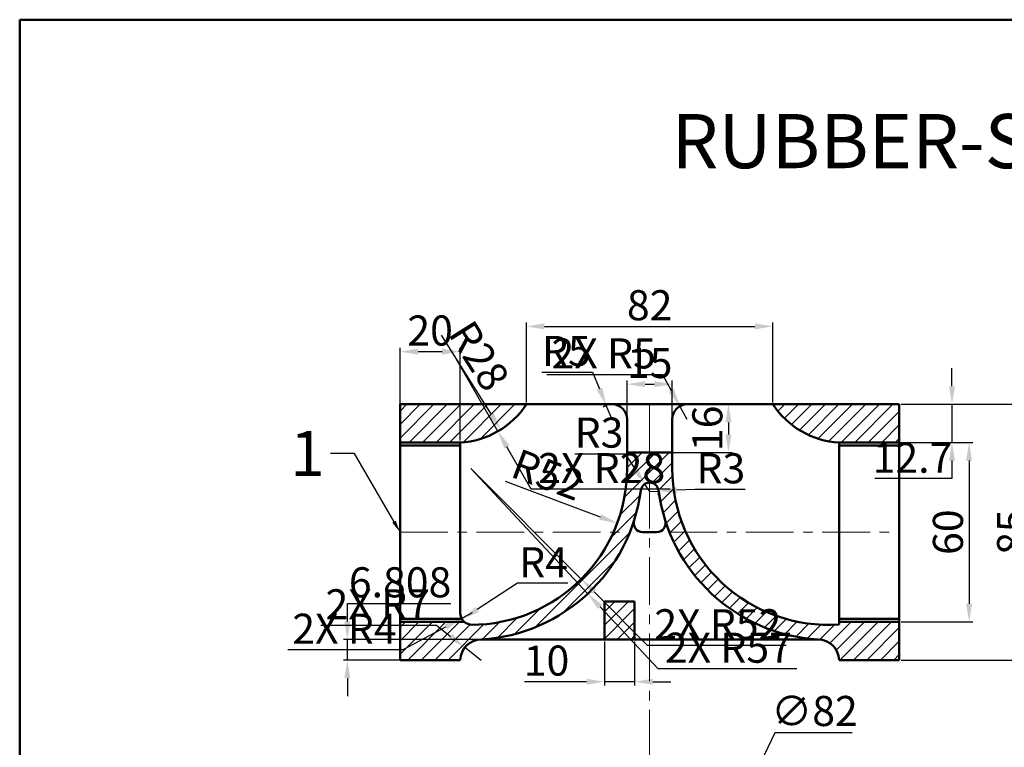
# Model space of a CAD drawing. Units: millimetres. Extents: x 147 to 984, y -369 to 435.
# Tile 5 of 10: x 147 to 475, y 193 to 435. Entities that reach past the tile are written whole.
import ezdxf
from ezdxf import colors
from ezdxf.entities.mleader import LeaderData, LeaderLine
from ezdxf.math import Vec2, Vec3

# ---------------------------------------------------------------- set-up
doc = ezdxf.new("R2010")
doc.units = ezdxf.units.MM
doc.header["$LTSCALE"] = 0.5
doc.linetypes.add('CENTER', pattern=[50.8, 31.75, -6.35, 6.35, -6.35])
for name, color, linetype, lineweight in [('M-CNTR', 1, 'CENTER', 18), ('M-DIMS', 2, 'Continuous', 25), ('M-HATC', 8, 'Continuous', 18), ('M-OUTL', 7, 'Continuous', 50), ('M-TEXT', 7, 'Continuous', 25)]:
    doc.layers.add(name, color=color, linetype=linetype, lineweight=lineweight)
doc.styles.get("Standard").update_dxf_attribs({"font": 'arial.ttf'})
doc.dimstyles.new('ISO-25', dxfattribs={"dimtxt": 10, "dimasz": 6, "dimexe": 1.25, "dimexo": 0.625, "dimtad": 1, "dimtoh": 1, "dimdec": 0, "dimtxsty": 'Standard', "dimcen": 2.5, "dimadec": 0, "dimazin": 0, "dimtfac": 1, "dimtdec": 0, "dimtmove": 0, "dimatfit": 3, "dimfxl": 1, "dimarcsym": 0})

# ---------------------------------------------------------------- blocks, each defined once
blk = doc.blocks.new('*D1')
at = {"layer": 'Defpoints', "color": 0, "transparency": 16777216}
for p in [(397.82, 333.39), (315.82, 307.49), (397.82, 307.49)]:
    blk.add_point(p, dxfattribs=at)
at = {"layer": 'M-DIMS', "color": 0, "lineweight": -2, "transparency": 16777216}
for p, q in [((315.82, 308.12), (315.82, 334.64)), ((397.82, 308.12), (397.82, 334.64)), ((321.82, 333.39), (391.82, 333.39))]:
    blk.add_line(p, q, dxfattribs=at)
at = {"layer": 'M-DIMS', "color": 0, "transparency": 16777216}
for points in [[(321.82, 334.39), (321.82, 332.39), (315.82, 333.39)], [(391.82, 334.39), (391.82, 332.39), (397.82, 333.39)]]:
    blk.add_solid(points, dxfattribs=at)
at = {"layer": 'M-DIMS', "color": 0, "transparency": 16777216, "insert": (356.82, 339.12), "char_height": 10, "attachment_point": 5}
blk.add_mtext('82', dxfattribs=at)
blk = doc.blocks.new('*D2')
at = {"layer": 'Defpoints', "color": 0, "transparency": 16777216}
for p in [(439.82, 307.49), (439.82, 222.49), (484.37, 222.49)]:
    blk.add_point(p, dxfattribs=at)
at = {"layer": 'M-DIMS', "color": 0, "lineweight": -2, "transparency": 16777216}
for p, q in [((440.44, 307.49), (485.62, 307.49)), ((484.37, 301.49), (484.37, 228.49)), ((440.44, 222.49), (485.62, 222.49))]:
    blk.add_line(p, q, dxfattribs=at)
at = {"layer": 'M-DIMS', "color": 0, "transparency": 16777216}
for points in [[(483.37, 301.49), (485.37, 301.49), (484.37, 307.49)], [(483.37, 228.49), (485.37, 228.49), (484.37, 222.49)]]:
    blk.add_solid(points, dxfattribs=at)
at = {"layer": 'M-DIMS', "color": 0, "transparency": 16777216, "insert": (478.64, 264.99), "char_height": 10, "attachment_point": 5, "rotation": 90}
blk.add_mtext('85', dxfattribs=at)
blk = doc.blocks.new('*D3')
at = {"layer": 'Defpoints', "color": 0, "transparency": 16777216}
for p in [(439.82, 294.79), (439.82, 235.19), (463.02, 235.19)]:
    blk.add_point(p, dxfattribs=at)
at = {"layer": 'M-DIMS', "color": 0, "lineweight": -2, "transparency": 16777216}
for p, q in [((440.44, 294.79), (464.27, 294.79)), ((463.02, 288.79), (463.02, 241.19)), ((440.44, 235.19), (464.27, 235.19))]:
    blk.add_line(p, q, dxfattribs=at)
at = {"layer": 'M-DIMS', "color": 0, "transparency": 16777216}
for points in [[(462.02, 288.79), (464.02, 288.79), (463.02, 294.79)], [(462.02, 241.19), (464.02, 241.19), (463.02, 235.19)]]:
    blk.add_solid(points, dxfattribs=at)
at = {"layer": 'M-DIMS', "color": 0, "transparency": 16777216, "insert": (457.29, 264.99), "char_height": 10, "attachment_point": 5, "rotation": 90}
blk.add_mtext('60', dxfattribs=at)
blk = doc.blocks.new('*D4')
at = {"layer": 'Defpoints', "color": 0, "transparency": 16777216}
for p in [(356.82, 307.49), (356.82, 291.49), (383.02, 291.49)]:
    blk.add_point(p, dxfattribs=at)
at = {"layer": 'M-DIMS', "color": 0, "lineweight": -2, "transparency": 16777216}
for p, q in [((357.44, 307.49), (384.27, 307.49)), ((383.02, 301.49), (383.02, 297.49)), ((357.44, 291.49), (384.27, 291.49))]:
    blk.add_line(p, q, dxfattribs=at)
at = {"layer": 'M-DIMS', "color": 0, "transparency": 16777216}
for points in [[(382.02, 301.49), (384.02, 301.49), (383.02, 307.49)], [(382.02, 297.49), (384.02, 297.49), (383.02, 291.49)]]:
    blk.add_solid(points, dxfattribs=at)
at = {"layer": 'M-DIMS', "color": 0, "transparency": 16777216, "insert": (377.29, 299.49), "char_height": 10, "attachment_point": 5, "rotation": 90}
blk.add_mtext('16', dxfattribs=at)
blk = doc.blocks.new('*D5')
at = {"layer": 'Defpoints', "color": 0, "transparency": 16777216}
for p in [(364.32, 314.17), (349.32, 296.22), (364.32, 296.22)]:
    blk.add_point(p, dxfattribs=at)
at = {"layer": 'M-DIMS', "color": 0, "lineweight": -2, "transparency": 16777216}
for p, q in [((349.32, 296.84), (349.32, 315.42)), ((364.32, 296.84), (364.32, 315.42)), ((355.32, 314.17), (358.32, 314.17))]:
    blk.add_line(p, q, dxfattribs=at)
at = {"layer": 'M-DIMS', "color": 0, "transparency": 16777216}
for points in [[(355.32, 315.17), (355.32, 313.17), (349.32, 314.17)], [(358.32, 315.17), (358.32, 313.17), (364.32, 314.17)]]:
    blk.add_solid(points, dxfattribs=at)
at = {"layer": 'M-DIMS', "color": 0, "transparency": 16777216, "insert": (356.82, 319.9), "char_height": 10, "attachment_point": 5}
blk.add_mtext('15', dxfattribs=at)
blk = doc.blocks.new('*D6')
at = {"layer": 'Defpoints', "color": 0, "transparency": 16777216}
for p in [(341.82, 229.3), (351.82, 229.3), (341.82, 215.28)]:
    blk.add_point(p, dxfattribs=at)
at = {"layer": 'M-DIMS', "color": 0, "lineweight": -2, "transparency": 16777216}
for p, q in [((341.82, 228.67), (341.82, 214.03)), ((351.82, 228.67), (351.82, 214.03)), ((335.82, 215.28), (315.22, 215.28)), ((351.82, 215.28), (341.82, 215.28)), ((357.82, 215.28), (363.82, 215.28))]:
    blk.add_line(p, q, dxfattribs=at)
at = {"layer": 'M-DIMS', "color": 0, "transparency": 16777216}
for points in [[(335.82, 216.28), (335.82, 214.28), (341.82, 215.28)], [(357.82, 216.28), (357.82, 214.28), (351.82, 215.28)]]:
    blk.add_solid(points, dxfattribs=at)
at = {"layer": 'M-DIMS', "color": 0, "transparency": 16777216, "insert": (322.52, 221.01), "char_height": 10, "attachment_point": 5}
blk.add_mtext('10', dxfattribs=at)
blk = doc.blocks.new('*D7')
at = {"layer": 'Defpoints', "color": 0, "transparency": 16777216}
for p in [(297.32, 286.19), (346.01, 267.94)]:
    blk.add_point(p, dxfattribs=at)
at = {"layer": 'M-DIMS', "color": 0, "lineweight": -2, "transparency": 16777216}
blk.add_line((308.75, 281.91), (340.39, 270.05), dxfattribs=at)
at = {"layer": 'M-DIMS', "color": 0, "transparency": 16777216}
blk.add_solid([(340.74, 270.99), (340.04, 269.11), (346.01, 267.94)], dxfattribs=at)
at = {"layer": 'M-DIMS', "color": 0, "transparency": 16777216, "insert": (322.49, 282.88), "char_height": 10, "attachment_point": 5, "rotation": 339.4574}
blk.add_mtext('R52', dxfattribs=at)
blk = doc.blocks.new('*D8')
at = {"layer": 'Defpoints', "color": 0, "transparency": 16777216}
for p in [(292.34, 322.75), (307.29, 299.07)]:
    blk.add_point(p, dxfattribs=at)
at = {"layer": 'M-DIMS', "color": 0, "lineweight": -2, "transparency": 16777216}
blk.add_line((287.45, 330.5), (304.08, 304.15), dxfattribs=at)
at = {"layer": 'M-DIMS', "color": 0, "transparency": 16777216}
blk.add_solid([(304.93, 304.68), (303.24, 303.61), (307.29, 299.07)], dxfattribs=at)
at = {"layer": 'M-DIMS', "color": 0, "transparency": 16777216, "insert": (299.01, 322.92), "char_height": 10, "attachment_point": 5, "rotation": 302.2569}
blk.add_mtext('R28', dxfattribs=at)
blk = doc.blocks.new('*D9')
at = {"layer": 'Defpoints', "color": 0, "transparency": 16777216}
for p in [(356.82, 278.46), (359.81, 278.61)]:
    blk.add_point(p, dxfattribs=at)
at = {"layer": 'M-DIMS', "color": 0, "lineweight": -2, "transparency": 16777216}
for p, q in [((356.82, 278.46), (359.81, 278.61)), ((371.8, 279.19), (365.81, 278.9)), ((388.55, 279.19), (371.8, 279.19))]:
    blk.add_line(p, q, dxfattribs=at)
blk.add_arc((356.82, 278.46), 3, 338.911, 7.402, dxfattribs=at)
at = {"layer": 'M-DIMS', "color": 0, "transparency": 16777216}
blk.add_solid([(365.76, 279.9), (365.86, 277.9), (359.81, 278.61)], dxfattribs=at)
at = {"layer": 'M-DIMS', "color": 0, "transparency": 16777216, "insert": (380.49, 284.92), "char_height": 10, "attachment_point": 5}
blk.add_mtext('R3', dxfattribs=at)
blk = doc.blocks.new('*D10')
at = {"layer": 'Defpoints', "color": 0, "transparency": 16777216}
for p in [(294.47, 236), (297.82, 238.19)]:
    blk.add_point(p, dxfattribs=at)
at = {"layer": 'M-DIMS', "color": 0, "lineweight": -2, "transparency": 16777216}
for p, q in [((312.86, 248.08), (299.49, 239.29)), ((329.57, 248.08), (312.86, 248.08))]:
    blk.add_line(p, q, dxfattribs=at)
at = {"layer": 'M-DIMS', "color": 0, "transparency": 16777216}
blk.add_solid([(298.94, 240.13), (300.04, 238.46), (294.47, 236)], dxfattribs=at)
at = {"layer": 'M-DIMS', "color": 0, "transparency": 16777216, "insert": (321.53, 253.7), "char_height": 10, "attachment_point": 5}
blk.add_mtext('R4', dxfattribs=at)
blk = doc.blocks.new('*D11')
at = {"layer": 'Defpoints', "color": 0, "transparency": 16777216}
for p in [(342.41, 307.11), (344.32, 302.49)]:
    blk.add_point(p, dxfattribs=at)
at = {"layer": 'M-DIMS', "color": 0, "lineweight": -2, "transparency": 16777216}
for p, q in [((321.01, 318.21), (337.84, 318.21)), ((337.84, 318.21), (340.13, 312.66)), ((344.32, 302.49), (342.41, 307.11))]:
    blk.add_line(p, q, dxfattribs=at)
blk.add_arc((344.32, 302.49), 5, 97.162, 126.7283, dxfattribs=at)
at = {"layer": 'M-DIMS', "color": 0, "transparency": 16777216}
blk.add_solid([(341.05, 313.04), (339.2, 312.28), (342.41, 307.11)], dxfattribs=at)
at = {"layer": 'M-DIMS', "color": 0, "transparency": 16777216, "insert": (329.11, 323.92), "char_height": 10, "attachment_point": 5}
blk.add_mtext('R5', dxfattribs=at)
blk = doc.blocks.new('*D26')
at = {"layer": 'Defpoints', "color": 0, "transparency": 16777216}
for p in [(374.55, 148.48), (339.08, 74.55)]:
    blk.add_point(p, dxfattribs=at)
at = {"layer": 'M-DIMS', "color": 0, "lineweight": -2, "transparency": 16777216}
for p, q in [((398.44, 198.26), (377.15, 153.89)), ((424.17, 198.26), (398.44, 198.26)), ((339.08, 74.55), (374.55, 148.48)), ((336.49, 69.14), (333.89, 63.73))]:
    blk.add_line(p, q, dxfattribs=at)
at = {"layer": 'M-DIMS', "color": 0, "transparency": 16777216}
for points in [[(376.25, 154.33), (378.05, 153.46), (374.55, 148.48)], [(335.58, 69.58), (337.39, 68.71), (339.08, 74.55)]]:
    blk.add_solid(points, dxfattribs=at)
at = {"layer": 'M-DIMS', "color": 0, "transparency": 16777216, "insert": (411.62, 204.27), "char_height": 10, "attachment_point": 5}
blk.add_mtext('∅82', dxfattribs=at)
blk = doc.blocks.new('*D146')
at = {"layer": 'Defpoints', "color": 0, "ltscale": 0.5, "transparency": 16777216}
for p in [(439.82, 307.49), (419.82, 294.79), (457.34, 294.79)]:
    blk.add_point(p, dxfattribs=at)
at = {"layer": 'M-DIMS', "color": 0, "lineweight": -2, "ltscale": 0.5, "transparency": 16777216}
for p, q in [((457.34, 313.49), (457.34, 319.49)), ((440.44, 307.49), (458.59, 307.49)), ((457.34, 307.49), (457.34, 294.79)), ((420.44, 294.79), (458.59, 294.79)), ((457.34, 288.79), (457.34, 282.79)), ((457.34, 282.79), (431.68, 282.79))]:
    blk.add_line(p, q, dxfattribs=at)
at = {"layer": 'M-DIMS', "color": 0, "ltscale": 0.5, "transparency": 16777216}
for points in [[(456.34, 313.49), (458.34, 313.49), (457.34, 307.49)], [(456.34, 288.79), (458.34, 288.79), (457.34, 294.79)]]:
    blk.add_solid(points, dxfattribs=at)
at = {"layer": 'M-DIMS', "color": 0, "ltscale": 0.5, "transparency": 16777216, "insert": (444.2, 288.44), "char_height": 10, "attachment_point": 5}
blk.add_mtext('12.7', dxfattribs=at)
blk = doc.blocks.new('*D147')
at = {"layer": 'Defpoints', "color": 0, "ltscale": 0.5, "transparency": 16777216}
for p in [(256.3, 229.3), (300.81, 229.3), (293.82, 222.49)]:
    blk.add_point(p, dxfattribs=at)
at = {"layer": 'M-DIMS', "color": 0, "lineweight": -2, "ltscale": 0.5, "transparency": 16777216}
for p, q in [((256.3, 235.3), (256.3, 241.3)), ((256.3, 241.3), (290.74, 241.3)), ((300.19, 229.3), (255.05, 229.3)), ((256.3, 222.49), (256.3, 229.3)), ((293.19, 222.49), (255.05, 222.49)), ((256.3, 216.49), (256.3, 210.49))]:
    blk.add_line(p, q, dxfattribs=at)
at = {"layer": 'M-DIMS', "color": 0, "ltscale": 0.5, "transparency": 16777216}
for points in [[(255.3, 235.3), (257.3, 235.3), (256.3, 229.3)], [(255.3, 216.49), (257.3, 216.49), (256.3, 222.49)]]:
    blk.add_solid(points, dxfattribs=at)
at = {"layer": 'M-DIMS', "color": 0, "ltscale": 0.5, "transparency": 16777216, "insert": (273.83, 247.03), "char_height": 10, "attachment_point": 5}
blk.add_mtext('6.808', dxfattribs=at)
blk = doc.blocks.new('*D148')
at = {"layer": 'Defpoints', "color": 0, "ltscale": 0.5, "transparency": 16777216}
for p in [(293.82, 324.99), (273.82, 294.79), (293.82, 294.79)]:
    blk.add_point(p, dxfattribs=at)
at = {"layer": 'M-DIMS', "color": 0, "lineweight": -2, "ltscale": 0.5, "transparency": 16777216}
for p, q in [((273.82, 295.42), (273.82, 326.24)), ((279.82, 324.99), (287.82, 324.99)), ((293.82, 295.42), (293.82, 326.24))]:
    blk.add_line(p, q, dxfattribs=at)
at = {"layer": 'M-DIMS', "color": 0, "ltscale": 0.5, "transparency": 16777216}
for points in [[(279.82, 325.99), (279.82, 323.99), (273.82, 324.99)], [(287.82, 325.99), (287.82, 323.99), (293.82, 324.99)]]:
    blk.add_solid(points, dxfattribs=at)
at = {"layer": 'M-DIMS', "color": 0, "ltscale": 0.5, "transparency": 16777216, "insert": (283.82, 330.72), "char_height": 10, "attachment_point": 5}
blk.add_mtext('20', dxfattribs=at)
blk = doc.blocks.new('*D150')
at = {"layer": 'Defpoints', "color": 0, "ltscale": 0.5, "transparency": 16777216}
for p in [(297.32, 286.19), (336.24, 244.54)]:
    blk.add_point(p, dxfattribs=at)
at = {"layer": 'M-DIMS', "color": 0, "lineweight": -2, "ltscale": 0.5, "transparency": 16777216}
for p, q in [((297.32, 286.19), (336.24, 244.54)), ((359.59, 219.56), (340.33, 240.16)), ((405.76, 219.56), (359.59, 219.56))]:
    blk.add_line(p, q, dxfattribs=at)
at = {"layer": 'M-DIMS', "color": 0, "ltscale": 0.5, "transparency": 16777216}
blk.add_solid([(341.06, 240.84), (339.6, 239.48), (336.24, 244.54)], dxfattribs=at)
at = {"layer": 'M-DIMS', "color": 0, "ltscale": 0.5, "transparency": 16777216, "insert": (382.99, 225.29), "char_height": 10, "attachment_point": 5}
blk.add_mtext('2X R57', dxfattribs=at)
blk = doc.blocks.new('*D151')
at = {"layer": 'Defpoints', "color": 0, "ltscale": 0.5, "transparency": 16777216}
for p in [(297.32, 286.19), (334.09, 249.42)]:
    blk.add_point(p, dxfattribs=at)
at = {"layer": 'M-DIMS', "color": 0, "lineweight": -2, "ltscale": 0.5, "transparency": 16777216}
for p, q in [((297.32, 286.19), (334.09, 249.42)), ((356.15, 227.36), (338.33, 245.18)), ((402.22, 227.36), (356.15, 227.36))]:
    blk.add_line(p, q, dxfattribs=at)
at = {"layer": 'M-DIMS', "color": 0, "ltscale": 0.5, "transparency": 16777216}
blk.add_solid([(339.04, 245.89), (337.62, 244.47), (334.09, 249.42)], dxfattribs=at)
at = {"layer": 'M-DIMS', "color": 0, "ltscale": 0.5, "transparency": 16777216, "insert": (379.5, 233.09), "char_height": 10, "attachment_point": 5}
blk.add_mtext('2X R52', dxfattribs=at)
blk = doc.blocks.new('*D152')
at = {"layer": 'Defpoints', "color": 0, "ltscale": 0.5, "transparency": 16777216}
for p in [(292.34, 322.75), (306.34, 298.5)]:
    blk.add_point(p, dxfattribs=at)
at = {"layer": 'M-DIMS', "color": 0, "lineweight": -2, "ltscale": 0.5, "transparency": 16777216}
for p, q in [((292.34, 322.75), (306.34, 298.5)), ((317.45, 279.27), (309.34, 293.31)), ((363.64, 279.27), (317.45, 279.27))]:
    blk.add_line(p, q, dxfattribs=at)
at = {"layer": 'M-DIMS', "color": 0, "ltscale": 0.5, "transparency": 16777216}
blk.add_solid([(310.21, 293.81), (308.47, 292.81), (306.34, 298.5)], dxfattribs=at)
at = {"layer": 'M-DIMS', "color": 0, "ltscale": 0.5, "transparency": 16777216, "insert": (340.86, 285), "char_height": 10, "attachment_point": 5}
blk.add_mtext('2X R28', dxfattribs=at)
blk = doc.blocks.new('*D153')
at = {"layer": 'Defpoints', "color": 0, "ltscale": 0.5, "transparency": 16777216}
for p in [(366.9, 306.87), (369.32, 302.49)]:
    blk.add_point(p, dxfattribs=at)
at = {"layer": 'M-DIMS', "color": 0, "lineweight": -2, "ltscale": 0.5, "transparency": 16777216}
for p, q in [((322.6, 317.37), (361.09, 317.37)), ((361.09, 317.37), (363.99, 312.12)), ((369.32, 302.49), (366.9, 306.87))]:
    blk.add_line(p, q, dxfattribs=at)
at = {"layer": 'M-DIMS', "color": 0, "ltscale": 0.5, "transparency": 16777216}
blk.add_solid([(364.87, 312.6), (363.12, 311.63), (366.9, 306.87)], dxfattribs=at)
at = {"layer": 'M-DIMS', "color": 0, "ltscale": 0.5, "transparency": 16777216, "insert": (341.53, 323.1), "char_height": 10, "attachment_point": 5}
blk.add_mtext('2X R5', dxfattribs=at)
blk = doc.blocks.new('*D154')
at = {"layer": 'Defpoints', "color": 0, "ltscale": 0.5, "transparency": 16777216}
for p in [(355.19, 280.98), (356.82, 278.46)]:
    blk.add_point(p, dxfattribs=at)
at = {"layer": 'M-DIMS', "color": 0, "lineweight": -2, "ltscale": 0.5, "transparency": 16777216}
for p, q in [((331.91, 291.05), (348.66, 291.05)), ((348.66, 291.05), (351.92, 286.01)), ((356.82, 278.46), (355.19, 280.98))]:
    blk.add_line(p, q, dxfattribs=at)
at = {"layer": 'M-DIMS', "color": 0, "ltscale": 0.5, "transparency": 16777216}
blk.add_solid([(352.76, 286.56), (351.08, 285.47), (355.19, 280.98)], dxfattribs=at)
at = {"layer": 'M-DIMS', "color": 0, "ltscale": 0.5, "transparency": 16777216, "insert": (339.97, 296.78), "char_height": 10, "attachment_point": 5}
blk.add_mtext('R3', dxfattribs=at)
blk = doc.blocks.new('*D155')
at = {"layer": 'Defpoints', "color": 0, "ltscale": 0.5, "transparency": 16777216}
for p in [(294.29, 236.31), (297.82, 238.19)]:
    blk.add_point(p, dxfattribs=at)
at = {"layer": 'M-DIMS', "color": 0, "lineweight": -2, "ltscale": 0.5, "transparency": 16777216}
for p, q in [((297.82, 238.19), (294.29, 236.31)), ((274.83, 225.95), (288.99, 233.49)), ((236.46, 225.95), (274.83, 225.95))]:
    blk.add_line(p, q, dxfattribs=at)
at = {"layer": 'M-DIMS', "color": 0, "ltscale": 0.5, "transparency": 16777216}
blk.add_solid([(288.52, 234.38), (289.46, 232.61), (294.29, 236.31)], dxfattribs=at)
at = {"layer": 'M-DIMS', "color": 0, "ltscale": 0.5, "transparency": 16777216, "insert": (255.33, 231.6), "char_height": 10, "attachment_point": 5}
blk.add_mtext('2X R4', dxfattribs=at)
blk = doc.blocks.new('*D156')
at = {"layer": 'Defpoints', "color": 0, "ltscale": 0.5, "transparency": 16777216}
for p in [(295.32, 226.64), (300.82, 222.3)]:
    blk.add_point(p, dxfattribs=at)
at = {"layer": 'M-DIMS', "color": 0, "lineweight": -2, "ltscale": 0.5, "transparency": 16777216}
for p, q in [((247.5, 234.08), (285.91, 234.08)), ((285.91, 234.08), (290.62, 230.36)), ((300.82, 222.3), (295.32, 226.64))]:
    blk.add_line(p, q, dxfattribs=at)
at = {"layer": 'M-DIMS', "color": 0, "ltscale": 0.5, "transparency": 16777216}
blk.add_solid([(291.24, 231.14), (290, 229.58), (295.32, 226.64)], dxfattribs=at)
at = {"layer": 'M-DIMS', "color": 0, "ltscale": 0.5, "transparency": 16777216, "insert": (266.39, 239.73), "char_height": 10, "attachment_point": 5}
blk.add_mtext('2X R7', dxfattribs=at)

msp = doc.modelspace()

# ---------------------------------------------------------------- hatches: boundary and pattern name
at = {"layer": 'M-HATC'}
h = msp.add_hatch(dxfattribs=at)
h.set_pattern_fill('ANSI31', color=256)
h.paths.add_polyline_path([(315.8179, 307.4916), (273.8179, 307.4916), (273.8179, 294.7916), (293.8179, 294.7916, 0.23985719)])
h.paths.add_polyline_path([(350.2288, 264.9916), (344.8001, 264.9916, -0.29309888), (297.8596, 234.1944, -0.18511355), (295.1751, 235.1916), (273.8179, 235.1916), (273.8179, 222.4916), (293.8179, 222.4916, -0.40607308), (300.8126, 229.2991), (300.8179, 229.2991, 0.28979332)])
h.paths.add_polyline_path([(356.8179, 291.4916), (349.3179, 291.4916), (349.3179, 286.1916, -0.10536872), (344.8001, 264.9916), (350.2288, 264.9916, 0.06305784), (353.8429, 278.8482, -0.37686161), (356.8179, 281.4618)])
h.paths.add_polyline_path([(364.3179, 286.1916), (364.3179, 291.4916), (356.8179, 291.4916), (356.8179, 281.4618, -0.37686161), (359.7929, 278.8482, 0.06305784), (363.407, 264.9916), (368.8357, 264.9916, -0.10536872)])
h.paths.add_polyline_path([(368.8357, 264.9916), (363.407, 264.9916, 0.28979332), (412.8179, 229.2991, -0.40629324), (419.8179, 222.4916), (439.8179, 222.4916), (439.8179, 235.1916), (419.8179, 235.1916), (419.8179, 234.3095, -0.31433682)])
h.paths.add_polyline_path([(439.8179, 307.4916), (397.8179, 307.4916, 0.23985719), (419.8179, 294.7916), (439.8179, 294.7916)])
h = msp.add_hatch(dxfattribs=at)
h.set_pattern_fill('ANSI31', color=256)
h.paths.add_polyline_path([(351.8186, 241.9706), (346.8186, 241.9706), (346.8186, 229.2991), (351.8186, 229.2991)])
h.paths.add_polyline_path([(346.8186, 241.9706), (341.8186, 241.9706), (341.8186, 229.2991), (346.8186, 229.2991)])

# ---------------------------------------------------------------- linework, layer by layer
at = {"layer": 'M-CNTR'}
for p, q in [((356.8179, 307.4916), (356.8179, 23.5276)), ((273.8179, 264.9916), (350.2288, 264.9916)), ((363.407, 264.9916), (439.8179, 264.9916))]:
    msp.add_line(p, q, dxfattribs=at)
at = {"layer": 'M-OUTL'}
for p, q in [((273.8179, 307.4916), (273.8179, 222.4916)), ((356.8179, 307.4916), (273.8179, 307.4916)), ((439.8179, 307.4916), (356.8179, 307.4916)), ((439.8179, 222.4916), (439.8179, 307.4916)), ((349.3179, 302.4916), (349.3179, 286.1916)), ((364.3179, 302.4916), (364.3179, 286.1916)), ((273.8179, 294.7916), (293.8179, 294.7916)), ((293.8179, 294.7916), (293.8179, 238.1942)), ((419.8179, 234.3095), (419.8179, 294.7916)), ((419.8179, 294.7916), (439.8179, 294.7916)), ((273.8179, 293.7916), (293.8179, 293.7916)), ((364.3179, 291.4916), (349.3179, 291.4916)), ((419.8179, 293.7916), (439.8179, 293.7916)), ((354.491, 264.9916), (359.1448, 264.9916)), ((341.8186, 229.2991), (341.8186, 241.9706)), ((341.8186, 241.9706), (351.8186, 241.9706)), ((351.8186, 229.2991), (351.8186, 241.9706)), ((273.8179, 236.1916), (294.3553, 236.1916)), ((419.8179, 236.1916), (439.8179, 236.1916)), ((273.8179, 235.1916), (295.1751, 235.1916)), ((419.8179, 235.1916), (439.8179, 235.1916)), ((412.8232, 229.2991), (300.8126, 229.2991)), ((273.8179, 222.4916), (293.8179, 222.4916)), ((419.8179, 222.4916), (439.8179, 222.4916))]:
    msp.add_line(p, q, dxfattribs=at)
at = {"layer": 'M-OUTL', "ltscale": 0.5}
msp.add_lwpolyline([(147.3511, 435.3078), (984.0884, 435.3078), (984.0884, -369.4968), (147.3511, -369.4968)], close=True, dxfattribs=at)
at = {"layer": 'M-OUTL'}
for centre, radius, start, end in [((292.3424, 322.7527), 28, 273.020675, 326.972661), ((344.3179, 302.4916), 5, 0, 90), ((369.3179, 302.4916), 5, 90, 180), ((421.2934, 322.7527), 28, 213.027339, 266.979325), ((297.3179, 286.1916), 52, 270, 0), ((416.3179, 286.1916), 52, 180, 273.859364), ((297.3179, 286.1916), 57, 273.520376, 352.598), ((356.8179, 278.4618), 3, 7.402, 172.598), ((416.3179, 286.1916), 57, 187.402, 266.479624), ((354.491, 267.9916), 3, 162.342079, 270), ((359.1448, 267.9916), 3, 270, 17.657921), ((297.8179, 238.1942), 4, 180, 270.596842), ((300.8153, 222.2991), 7, 89.978344, 178.424643), ((412.8206, 222.2991), 7, 1.575357, 90.021656)]:
    msp.add_arc(centre, radius, start, end, dxfattribs=at)

# ---------------------------------------------------------------- texts
at = {"layer": 'M-TEXT', "ltscale": 0.5, "insert": (313.9939, 403.9552), "char_height": 18, "attachment_point": 1}
msp.add_mtext_dynamic_manual_height_columns('\\pxqc;RUBBER-SEATED VALVE ASSEMBLY', width=497.441574, gutter_width=12.5, heights=[0], dxfattribs=at)

# ---------------------------------------------------------------- dimensions: what is measured, and where the dimension line sits
at = {"layer": 'M-DIMS'}
for base, p1, p2, picture, middle in [((397.8179, 333.3876), (315.8179, 307.4916), (397.8179, 307.4916), '*D1', (356.8179, 339.1183)), ((364.3179, 314.1693), (349.3179, 296.2182), (364.3179, 296.2182), '*D5', (356.8179, 319.9)), ((341.8186, 215.2842), (351.8186, 229.2991), (341.8186, 229.2991), '*D6', (322.519, 221.015))]:
    dim = msp.add_linear_dim(base=base, p1=p1, p2=p2, dimstyle='ISO-25', override={"dimclrd": 0, "dimclre": 0, "dimclrt": 0}, dxfattribs=at)
    dim.commit()
    dim.dimension.update_dxf_attribs({"geometry": picture, "text_midpoint": middle})
at = {"layer": 'M-DIMS', "ltscale": 0.5}
dim = msp.add_linear_dim(base=(293.8179, 324.9916), p1=(273.8179, 294.7916), p2=(293.8179, 294.7916), dimstyle='ISO-25', override={"dimdec": 0, "dimlfac": 1, "dimrnd": 0, "dimzin": 0, "dimdsep": 46, "dimlunit": 2}, dxfattribs=at)
dim.commit()
dim.dimension.update_dxf_attribs({"geometry": '*D148', "text_midpoint": (283.8179, 330.7223)})
for center, mpoint, picture, middle in [((369.3179, 302.4916), (366.8972, 306.8665), '*D153', (341.5335, 323.0971)), ((292.3424, 322.7527), (306.3409, 298.5031), '*D152', (340.857, 284.9975)), ((300.8153, 222.2991), (295.3234, 226.6396), '*D156', (266.3922, 239.7292)), ((297.8179, 238.1942), (294.2873, 236.314), '*D155', (255.3311, 231.5993))]:
    dim = msp.add_radius_dim(center=center, mpoint=mpoint, text='2X <>', dimstyle='ISO-25', override={"dimdec": 0, "dimlfac": 1, "dimrnd": 0, "dimzin": 0, "dimdsep": 46, "dimlunit": 2}, dxfattribs=at)
    dim.commit()
    dim.dimension.update_dxf_attribs({"geometry": picture, "text_midpoint": middle})
at = {"layer": 'M-DIMS'}
for center, mpoint, picture, middle in [((292.3424, 322.7527), (307.2865, 299.0741), '*D8', (294.1663, 319.8628)), ((297.3179, 286.1916), (346.0113, 267.9446), '*D7', (320.4761, 277.5134)), ((297.8179, 238.1942), (294.4747, 235.998), '*D10', (321.5294, 248.077))]:
    dim = msp.add_radius_dim(center=center, mpoint=mpoint, dimstyle='ISO-25', override={"dimclrd": 0, "dimclre": 0, "dimclrt": 0}, dxfattribs=at)
    dim.commit()
    dim.dimension.update_dxf_attribs({"geometry": picture, "text_midpoint": middle, "dimtype": 164})
for center, mpoint, picture, middle in [((344.3179, 302.4916), (342.4122, 307.1142), '*D11', (329.1132, 323.9186)), ((356.8179, 278.4618), (359.8144, 278.6075), '*D9', (380.488, 284.9245))]:
    dim = msp.add_radius_dim(center=center, mpoint=mpoint, dimstyle='ISO-25', override={"dimclrd": 0, "dimclre": 0, "dimclrt": 0}, dxfattribs=at)
    dim.commit()
    dim.dimension.update_dxf_attribs({"geometry": picture, "text_midpoint": middle})
at = {"layer": 'M-DIMS', "ltscale": 0.5}
for base, p1, p2, override, picture, middle in [((457.3399, 294.7916), (439.8179, 307.4916), (419.8179, 294.7916), {"dimdec": 1, "dimlfac": 1, "dimrnd": 0, "dimzin": 0, "dimdsep": 46, "dimlunit": 2}, '*D146', (444.1979, 288.437)), ((256.29587, 229.29912), (293.81791, 222.49157), (300.81261, 229.29912), {"dimdec": 3, "dimlfac": 1, "dimrnd": 0, "dimzin": 0, "dimdsep": 46, "dimlunit": 2}, '*D147', (273.83083, 247.02985))]:
    dim = msp.add_linear_dim(base=base, p1=p1, p2=p2, angle=90, dimstyle='ISO-25', override=override, dxfattribs=at)
    dim.commit()
    dim.dimension.update_dxf_attribs({"geometry": picture, "text_midpoint": middle})
at = {"layer": 'M-DIMS'}
dim = msp.add_linear_dim(base=(383.02, 291.4916), p1=(356.8179, 307.4916), p2=(356.8179, 291.4916), angle=90, dimstyle='ISO-25', override={"dimclrd": 0, "dimclre": 0, "dimclrt": 0}, dxfattribs=at)
dim.commit()
dim.dimension.update_dxf_attribs({"geometry": '*D4', "text_midpoint": (377.2893, 299.4916)})
for p1, p2, distance, picture, middle in [((439.8179, 307.4916), (439.8179, 222.4916), 44.551, '*D2', (478.6381, 264.9916)), ((439.8179, 294.7916), (439.8179, 235.1916), 23.2015, '*D3', (457.2887, 264.9916))]:
    dim = msp.add_aligned_dim(p1=p1, p2=p2, distance=distance, dimstyle='ISO-25', override={"dimclrd": 0, "dimclre": 0, "dimclrt": 0}, dxfattribs=at)
    dim.commit()
    dim.dimension.update_dxf_attribs({"geometry": picture, "text_midpoint": middle})
at = {"layer": 'M-DIMS', "ltscale": 0.5}
dim = msp.add_radius_dim(center=(356.8179, 278.4618), mpoint=(355.186, 280.9791), dimstyle='ISO-25', override={"dimdec": 0, "dimlfac": 1, "dimrnd": 0, "dimzin": 0, "dimdsep": 46, "dimlunit": 2}, dxfattribs=at)
dim.commit()
dim.dimension.update_dxf_attribs({"geometry": '*D154', "text_midpoint": (339.9706, 296.7824)})
for mpoint, picture, middle in [((336.2351, 244.5448), '*D150', (382.9867, 219.5568)), ((334.0872, 249.4218), '*D151', (379.4989, 227.3599))]:
    dim = msp.add_radius_dim(center=(297.3179, 286.1916), mpoint=mpoint, text='2X <>', dimstyle='ISO-25', override={"dimdec": 0, "dimlfac": 1, "dimrnd": 0, "dimzin": 0, "dimdsep": 46, "dimlunit": 2}, dxfattribs=at)
    dim.commit()
    dim.dimension.update_dxf_attribs({"geometry": picture, "text_midpoint": middle, "dimtype": 164})
at = {"layer": 'M-DIMS'}
dim = msp.add_diameter_dim_2p(p1=(339.0816, 74.553), p2=(374.5542, 148.4833), dimstyle='ISO-25', override={"dimclrd": 0, "dimclre": 0, "dimclrt": 0}, dxfattribs=at)
dim.commit()
dim.dimension.update_dxf_attribs({"geometry": '*D26', "text_midpoint": (411.6154, 198.2633), "dimtype": 163})

# ---------------------------------------------------------------- leaders
at = {"layer": 'M-TEXT'}
ml = msp.add_multileader_mtext('Standard', dxfattribs=at)
ml.set_content('1', color=256)
ml.set_leader_properties()
ml.build(insert=Vec2(0, 0))
ctx = ml.context
ctx.base_point, ctx.char_height, ctx.plane_origin = Vec3(241.1824, 291.1633), 15, Vec3(273.8179, 264.9916)
ctx.text_align_type = 2
notes = []
notes.append((ctx, [(0, (1, 1, 0), (258.7077, 291.1633), (-1, 0), 8, [(0, [(273.8179, 264.9916)], 0, [])])]))
ctx.mtext.insert, ctx.mtext.alignment, ctx.mtext.flow_direction = Vec3(248.7077, 298.6633), 3, 5
for ctx, leaders in notes:
    for number, flags, end, landing, length, lines in leaders:
        leader = LeaderData()
        leader.index, (leader.has_last_leader_line, leader.has_dogleg_vector, leader.attachment_direction) = number, flags
        leader.last_leader_point, leader.dogleg_vector, leader.dogleg_length = Vec3(end), Vec3(landing), length
        for number, points, colour, breaks in lines:
            line = LeaderLine()
            line.index, line.vertices, line.color, line.breaks = number, Vec3.list(points), colors.encode_raw_color(colour), breaks
            leader.lines.append(line)
        ctx.leaders.append(leader)

doc.saveas('drawing.dxf')
